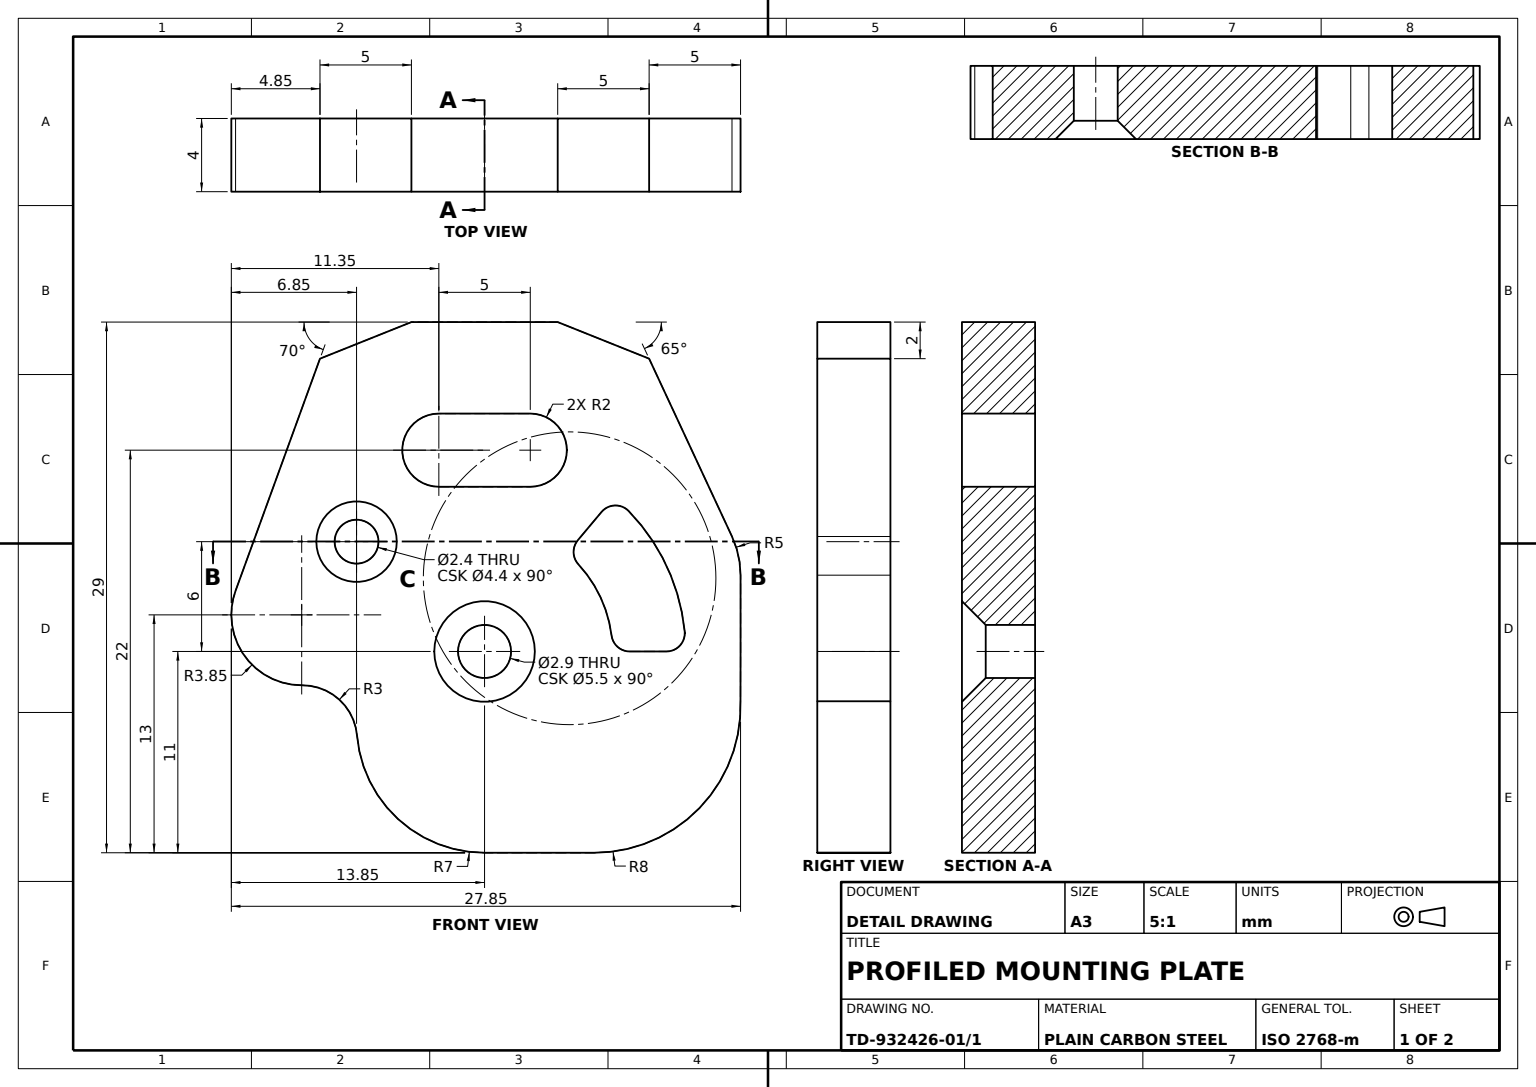
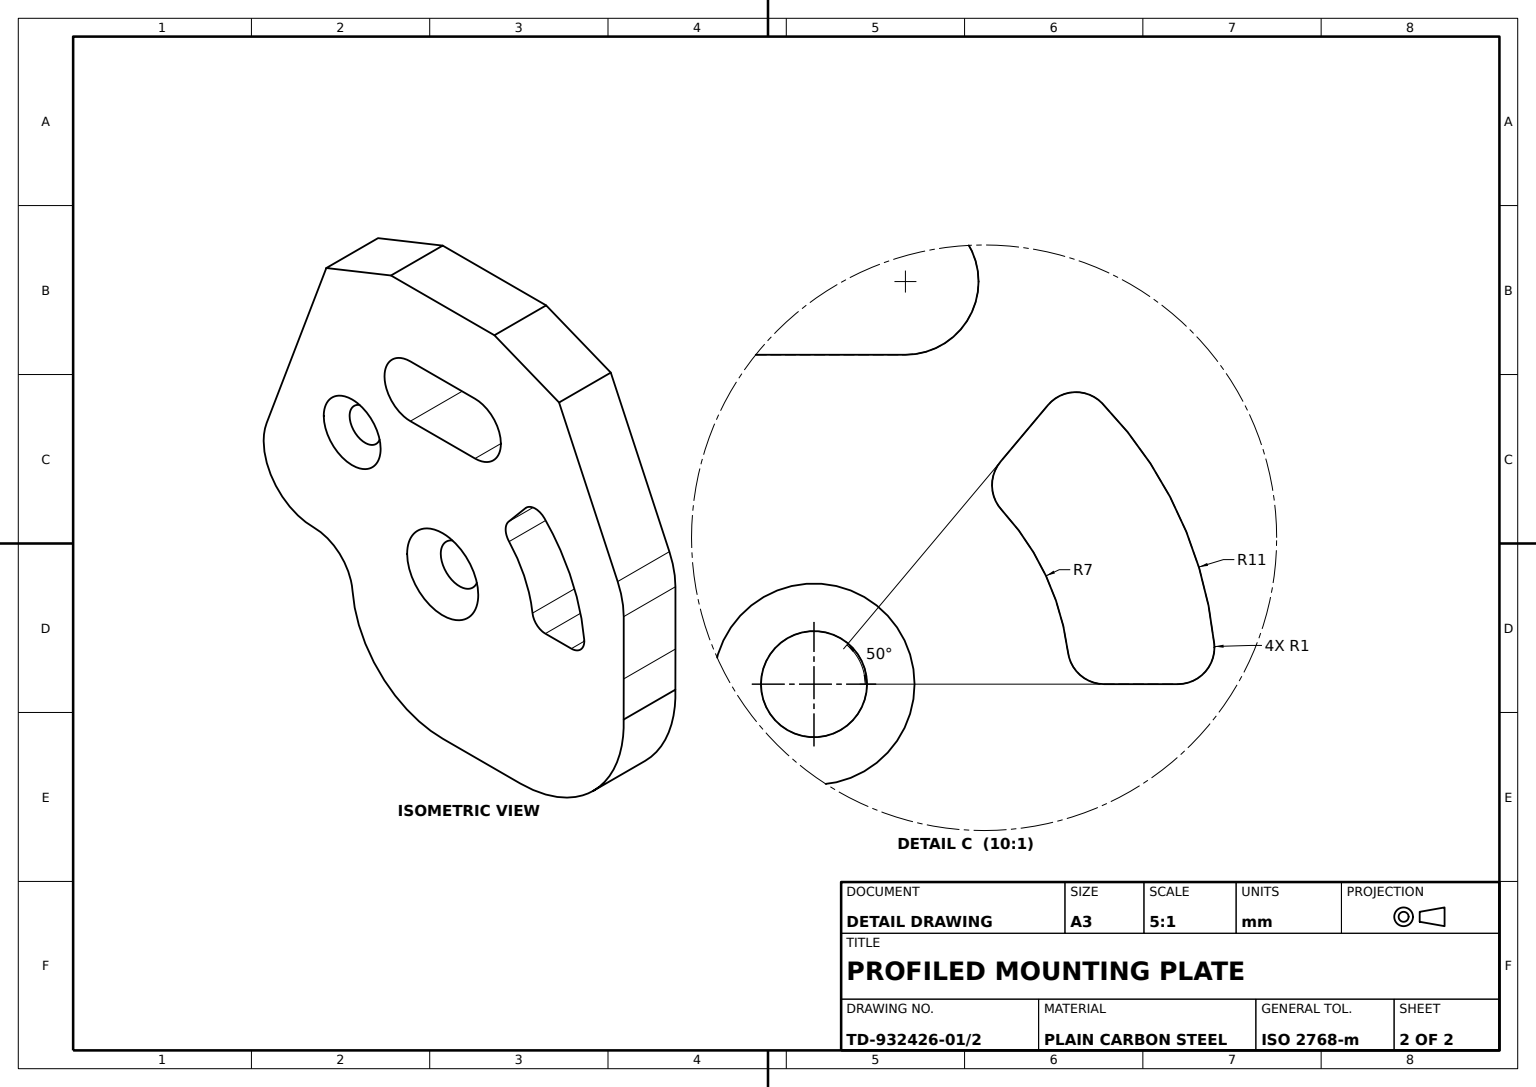
SolidWorks part; units mm, degrees
material "Plain Carbon Steel"
ref_plane "Front Plane" through (0, 0, 0) normal (0, 0, 1) x (1, 0, 0)
ref_plane "Top Plane" through (0, 0, 0) normal (0, 1, 0) x (1, 0, 0)
ref_plane "Right Plane" through (0, 0, 0) normal (1, 0, 0) x (0, 0, -1)
sketch "Cam Plate Profile Sketch" plane through (0, 0, 0) normal (0, 0, 1) x (1, 0, 0)
  line L0 (0, 0) -> (0, 4.4742) construction
  line L1 (4, 4.4742) -> (-4, 4.4742)
  line L2 (-4, 4.4742) -> (-9, 2.4742)
  line L3 (-9, 2.4742) -> (-13.6165, -10.2095)
  line L4 (-9, 2.4742) -> (-26.7983, 2.4742) construction
  line L5 (4, 4.4742) -> (9, 2.4742)
  line L6 (9, 2.4742) -> (25.7647, 2.4742) construction
  line L7 (9, 2.4742) -> (13.5315, -7.2437)
  line L8 (14, -9.3568) -> (14, -13.5258)
  line L9 (0, 4.4742) -> (0, -13.5258) construction
  line L10 (0, -13.5258) -> (24.6853, -13.5258) construction
  line L11 (-31.6272, -11.5258) -> (-10, -11.5258) construction
  line L12 (0, -13.5258) -> (0, -24.5258) construction
  line L13 (0, -24.5258) -> (6, -24.5258)
  line L14 (14, -13.5258) -> (13.9951, -16.2472)
  arc A0 (13.5315, -7.2437) -> (14, -9.3568) centre (9, -9.3568) cw
  circle A1 centre (0, -13.5258) radius 9 construction
  arc A3 (-13.6165, -10.2095) -> (-9.9798, -15.3743) centre (-10, -11.5258) ccw
  arc A4 (-6.9748, -18.1197) -> (0, -24.5258) centre (0, -17.5258) ccw
  arc A5 (-6.9748, -18.1197) -> (-9.9798, -15.3743) centre (-9.964, -18.3743) ccw
  arc A6 (13.9951, -16.2472) -> (6, -24.5258) centre (6, -16.5258) cw
  point P6 (0, 4.4742)
  point P15 (14, -8.2483)
  dimension "D8" = 5
  dimension "D12" = 4.4742
  dimension "D14" = 18
  dimension "D15" = 8
  dimension "D17" = 16.7647
  dimension "D4" = 70
  dimension "D16" = 7
  dimension "D1" = 8
  dimension "D2" = 5
  dimension "D3" = 2
  dimension "D5" = 2
  dimension "D6" = 65
  dimension "D7" = 14
  dimension "D9" = 18
  dimension "D10" = 10
  dimension "D11" = 2
  dimension "D13" = 11
  dimension "D18" = 17.7983
  dimension "D19" = 21.6272
  dimension "D20" = 24.6853
  dimension "D21" = 9.964
  dimension "D22" = 2.7214
extrude "Cam Plate 4mm" add sketch "Cam Plate Profile Sketch" along normal blind 4
sketch "Slot Profiles Sketch" plane through (0, 0, 4) normal (0, 0, 1) x (1, 0, 0)
  line L0 (-2.5, -2.5258) -> (2.5, -2.5258) construction
  line L1 (-2.5, -0.5258) -> (2.5, -0.5258)
  line L2 (-2.5, -4.5258) -> (2.5, -4.5258)
  line L3 (4, 4.4742) -> (-4, 4.4742) construction
  line L4 (5.102, -7.4455) -> (6.3957, -5.9037)
  line L5 (0, -13.5258) -> (30.2881, -13.5258) construction
  line L6 (7.9373, -13.5258) -> (9.9499, -13.5258)
  arc A0 (-2.5, -0.5258) -> (-2.5, -4.5258) centre (-2.5, -2.5258) ccw
  arc A1 (2.5, -4.5258) -> (2.5, -0.5258) centre (2.5, -2.5258) ccw
  arc A2 (9, -13.5258) -> (5.7851, -6.6314) centre (0, -13.5258) ccw construction
  arc A3 (6.9451, -12.6508) -> (5.1345, -8.7679) centre (0, -13.5258) ccw
  arc A4 (10.9449, -12.4258) -> (7.8779, -5.8486) centre (0, -13.5258) ccw
  arc A5 (9.9499, -13.5258) -> (10.9449, -12.4258) centre (9.9499, -12.5258) ccw
  arc A6 (7.9373, -13.5258) -> (6.9451, -12.6508) centre (7.9373, -12.5258) cw
  arc A7 (5.102, -7.4455) -> (5.1345, -8.7679) centre (5.868, -8.0883) ccw
  arc A8 (6.3957, -5.9037) -> (7.8779, -5.8486) centre (7.1617, -6.5465) cw
  point P2 (0, -2.5258)
  point P8 (0, -4.5258)
  point P21 (11, -13.5258)
  point P24 (7, -13.5258)
  point P27 (4.4995, -8.1634)
  point P30 (7.0707, -5.0993)
  dimension "D3" = 18
  dimension "D4" = 18
  dimension "D5" = 50
  dimension "D7" = 1
  dimension "D1" = 5
  dimension "D2" = 4
  dimension "D6" = 4
extrude "Slots Cut" cut sketch "Slot Profiles Sketch" against normal blind 4
sketch "M2.5 CSK Hole Location" plane through (0, 0, 4) normal (0, 0, 1) x (1, 0, 0)
  line L0 (0, 4.4742) -> (0, -13.5258) construction
  line L1 (4, 4.4742) -> (-4, 4.4742) construction
  line L2 (0, -13.5258) -> (-7, -13.5258) construction
  dimension "D1" = 7
  dimension "D2" = 18
hole_wizard "CSK Hole M2.5" positions "3DSketch2" profile "Sketch5" countersink size "M2.5" standard "ISO"
sketch3d "3DSketch2"
  point P0 (0, -13.5258, 4)
sketch "Sketch5" plane through (0, -13.5258, 4) normal (1, 0, 0) x (0, -1, 0)
  line L0 (0, 0) -> (0, 29.8712)
  line L1 (0, 29.8712) -> (1.45, 29)
  line L2 (1.45, 29) -> (1.45, 1.3)
  line L3 (1.45, 1.3) -> (2.75, 0)
  line L5 (2.75, 0) -> (0, 0)
  line L6 (-1.45, 1.3) -> (-2.75, 0) construction
  line L10 (0, 29.8712) -> (-1.45, 29) construction
  line L11 (0, -6.35) -> (0, 107.95) construction
  dimension "Hole Dia." = 2.9
  dimension "Hole Depth" = 29
  dimension "Near C'Sink Dia." = 5.5
  dimension "Near C'Sink Angle" = 90
  dimension "Drill Angle" = 118
sketch "M2 CSK Hole Location" plane through (0, 0, 4) normal (0, 0, 1) x (1, 0, 0)
  line L0 (0, -13.5258) -> (-7, -13.5258) construction
  line L1 (-7, -13.5258) -> (-7, -7.5258) construction
  dimension "D1" = 7
  dimension "D2" = 6
hole_wizard "CSK Hole M2" positions "3DSketch3" profile "Sketch7" countersink size "M2" standard "ISO"
sketch3d "3DSketch3"
  point P0 (-7, -7.5258, 4)
sketch "Sketch7" plane through (-7, -7.5258, 4) normal (1, 0, 0) x (0, -1, 0)
  line L0 (0, 0) -> (0, 29.721)
  line L1 (0, 29.721) -> (1.2, 29)
  line L2 (1.2, 29) -> (1.2, 1)
  line L3 (1.2, 1) -> (2.2, 0)
  line L5 (2.2, 0) -> (0, 0)
  line L6 (-1.2, 1) -> (-2.2, 0) construction
  line L10 (0, 29.721) -> (-1.2, 29) construction
  line L11 (0, -6.35) -> (0, 107.95) construction
  dimension "Hole Dia." = 2.4
  dimension "Hole Depth" = 29
  dimension "Near C'Sink Dia." = 4.4
  dimension "Near C'Sink Angle" = 90
  dimension "Drill Angle" = 118
